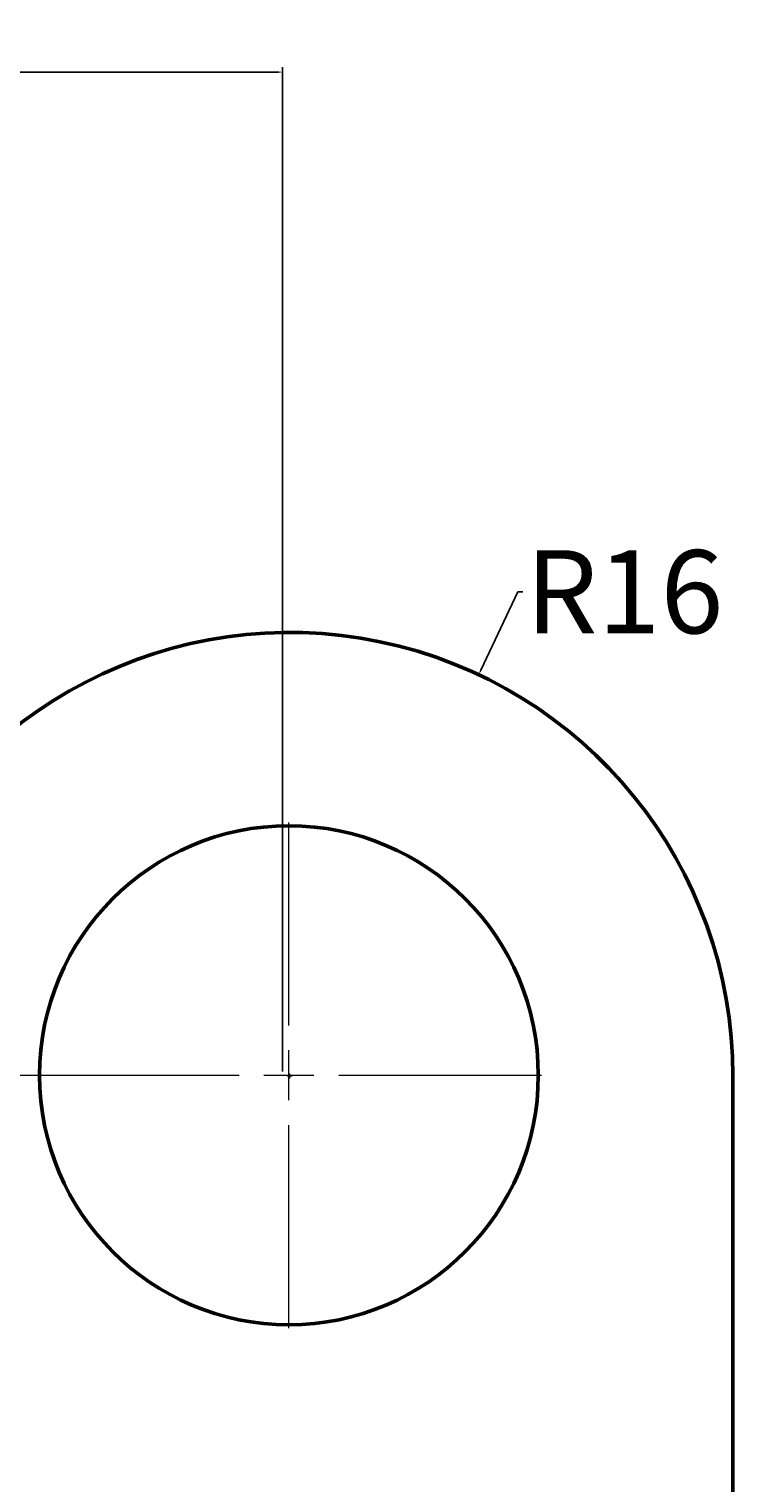
# Model space of a CAD drawing. Units: millimetres. Extents: x -50 to 109, y -46 to 152.
# Tile 18 of 18: x 62 to 87, y 100 to 152. Entities that reach past the tile are written whole.
import ezdxf

# ---------------------------------------------------------------- set-up
doc = ezdxf.new("R2010")
doc.units = ezdxf.units.MM
doc.header["$MEASUREMENT"] = 0
doc.linetypes.add('CENTER', pattern=[50.8, 31.75, -6.35, 6.35, -6.35])
for name, color, linetype, lineweight in [('M-CNTR', 1, 'CENTER', 18), ('M-DIMS', 2, 'Continuous', 25), ('M-OUTL', 7, 'Continuous', 50)]:
    doc.layers.add(name, color=color, linetype=linetype, lineweight=lineweight)
doc.styles.get("Standard").update_dxf_attribs({"font": 'arial.ttf'})
doc.dimstyles.get("Standard").update_dxf_attribs({"dimtxt": 0.18, "dimasz": 0.18, "dimexe": 0.18, "dimexo": 0.0625, "dimgap": 0.09, "dimtad": 0, "dimtih": 1, "dimtoh": 1, "dimdec": 4, "dimzin": 0, "dimdsep": 46, "dimtxsty": 'Standard', "dimcen": 0.09, "dimadec": 0, "dimazin": 0, "dimtfac": 1, "dimtdec": 4, "dimtofl": 0, "dimtmove": 0, "dimatfit": 3, "dimfxl": 1, "dimtolj": 1, "dimtzin": 0, "dimarcsym": 0})

# ---------------------------------------------------------------- blocks, each defined once
blk = doc.blocks.new('*U4')
at = {"layer": 'M-CNTR', "color": 0, "transparency": 16777216}
for p, q in [((0, 1.8), (0, 9.12)), ((-18.399, 0), (-1.8, 0)), ((1.8, 0), (9.12, 0)), ((0, -9.12), (0, -1.8))]:
    blk.add_line(p, q, dxfattribs=at)
at = {"layer": 'M-CNTR', "color": 0, "linetype": 'Continuous', "transparency": 16777216}
for p, q in [((0, -0.9), (0, 0.9)), ((-0.9, 0), (0.9, 0))]:
    blk.add_line(p, q, dxfattribs=at)
blk = doc.blocks.new('*D7')
at = {"layer": 'Defpoints', "color": 0, "transparency": 16777216}
for p in [(70.892, 150.415), (-5.074, 114.299), (70.892, 114.299)]:
    blk.add_point(p, dxfattribs=at)
at = {"layer": 'M-DIMS', "color": 0, "lineweight": -2, "transparency": 16777216}
for p, q in [((-5.074, 114.361), (-5.074, 150.595)), ((70.892, 114.361), (70.892, 150.595)), ((-4.894, 150.415), (30.684, 150.415)), ((70.712, 150.415), (35.134, 150.415))]:
    blk.add_line(p, q, dxfattribs=at)
at = {"layer": 'M-DIMS', "color": 0, "transparency": 16777216}
for points in [[(-4.894, 150.445), (-4.894, 150.385), (-5.074, 150.415)], [(70.712, 150.445), (70.712, 150.385), (70.892, 150.415)]]:
    blk.add_solid(points, dxfattribs=at)
at = {"layer": 'M-DIMS', "color": 0, "transparency": 16777216, "insert": (32.909, 150.415), "char_height": 0.18, "attachment_point": 5}
blk.add_mtext('\\A1;{\\H16.66667x;76}', dxfattribs=at)
blk = doc.blocks.new('*D8')
at = {"layer": 'Defpoints', "color": 0, "transparency": 16777216}
for p in [(77.967, 128.678), (71.145, 114.206)]:
    blk.add_point(p, dxfattribs=at)
at = {"layer": 'M-DIMS', "color": 0, "lineweight": -2, "transparency": 16777216}
for p, q in [((79.378, 131.671), (78.044, 128.841)), ((79.558, 131.671), (79.378, 131.671)), ((71.055, 114.206), (71.235, 114.206)), ((71.145, 114.116), (71.145, 114.296))]:
    blk.add_line(p, q, dxfattribs=at)
at = {"layer": 'M-DIMS', "color": 0, "transparency": 16777216}
blk.add_solid([(78.017, 128.854), (78.071, 128.828), (77.967, 128.678)], dxfattribs=at)
at = {"layer": 'M-DIMS', "color": 0, "transparency": 16777216, "insert": (83.231, 131.671), "char_height": 0.18, "attachment_point": 5}
blk.add_mtext('\\A1;{\\H16.66667x;R16}', dxfattribs=at)

msp = doc.modelspace()

# ---------------------------------------------------------------- linework, layer by layer
at = {"layer": 'M-OUTL'}
msp.add_line((87.1447, 114.19973), (87.12678, 66.54447), dxfattribs=at)
msp.add_circle((71.11949, 114.23094), 9, dxfattribs=at)
msp.add_arc((71.1447, 114.20575), 16, 359.978447, 156.508505, dxfattribs=at)

# ---------------------------------------------------------------- block references
at = {"layer": 'M-CNTR'}
msp.add_blockref('*U4', (71.11949, 114.23094), dxfattribs=at)

# ---------------------------------------------------------------- dimensions: what is measured, and where the dimension line sits
at = {"layer": 'M-DIMS'}
dim = msp.add_linear_dim(base=(70.89158, 150.41471), p1=(-5.07376, 114.29893), p2=(70.89158, 114.29893), text='{\\H16.66667x;76}', dimstyle='Standard', override={"dimclrd": 0, "dimclre": 0, "dimclrt": 0}, dxfattribs=at)
dim.commit()
dim.dimension.update_dxf_attribs({"geometry": '*D7', "text_midpoint": (32.90891, 150.41471)})
dim = msp.add_radius_dim(center=(71.1447, 114.20575), mpoint=(77.96714, 128.67828), text='{\\H16.66667x;R16}', dimstyle='Standard', override={"dimclrd": 0, "dimclre": 0, "dimclrt": 0}, dxfattribs=at)
dim.commit()
dim.dimension.update_dxf_attribs({"geometry": '*D8', "text_midpoint": (83.23112, 131.67094), "dimtype": 164})

doc.saveas('drawing.dxf')
